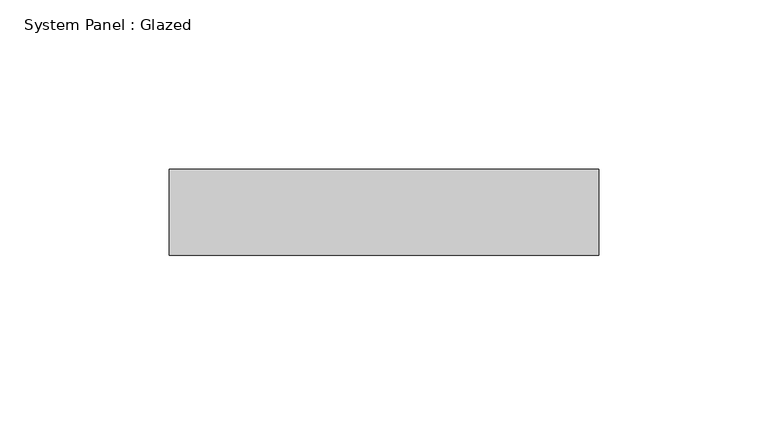
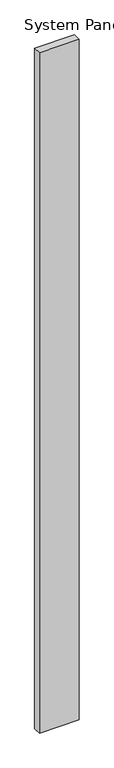
"""IFC4 building model written with IfcOpenShell, lengths in millimetres: plate geometry, System Panel : Glazed."""

from ifc_helpers import new_model, si_unit, origin, origin_with_axes, place, context, project, spatial, polyline, outline, extrude, source, transform, mapped, element, save


def system_panel_glazed_eef689be(model_context):
    return source(origin(), model_context, "Body", "SweptSolid", [
        extrude(outline(polyline([(63.5, 19.05), (-63.5, 19.05), (-63.5, 44.45), (63.5, 44.45), (63.5, 19.05)])), origin_with_axes(), (0.0, 0.0, 1.0), 2287.5875),
    ])


if __name__ == "__main__":
    model = new_model("IFC4")
    model_context = context("Model", 3, world=origin())
    ifc_project = project(units=[si_unit("LENGTHUNIT", "METRE", prefix="MILLI")], contexts=[model_context])
    site = spatial("IfcSite", under=ifc_project)
    building = spatial("IfcBuilding", under=site)
    placement = place(None, origin())
    system_panel_glazed_shape = system_panel_glazed_eef689be(model_context)
    element("IfcPlate", 1, ObjectType="System Panel : Glazed", at=placement, inside=building, context=model_context, shape_type="MappedRepresentation", body=[
        mapped(system_panel_glazed_shape, transform((0.0, 0.0, 0.0), x_axis=(1.0, 0.0, 0.0), y_axis=(0.0, 1.0, 0.0), z_axis=(0.0, 0.0, 1.0))),
    ])
    save(model, "model.ifc")

# Revit data of these elements
# Type "System Panel : Glazed"
#   Construction Type Id = "GSP4R"
#   Analytic Construction = "1/8 in Pilkington single glazing"
#   Visual Light Transmittance = 0.9
#   Solar Heat Gain Coefficient = 0.86
#   Heat Transfer Coefficient (U) = 1.18115 BTU/(h·ft²·°F)
#   Define Thermal Properties by = 1
# Element 1 (IfcPlate, "System Panel : Glazed")
#   Materials on its faces: "Glass"
# Materials
#   "Glass": class "Glass", colour RGB 0 128 192, transparency 0.75, Description = "Soda Lime Glass", Cost = 0
